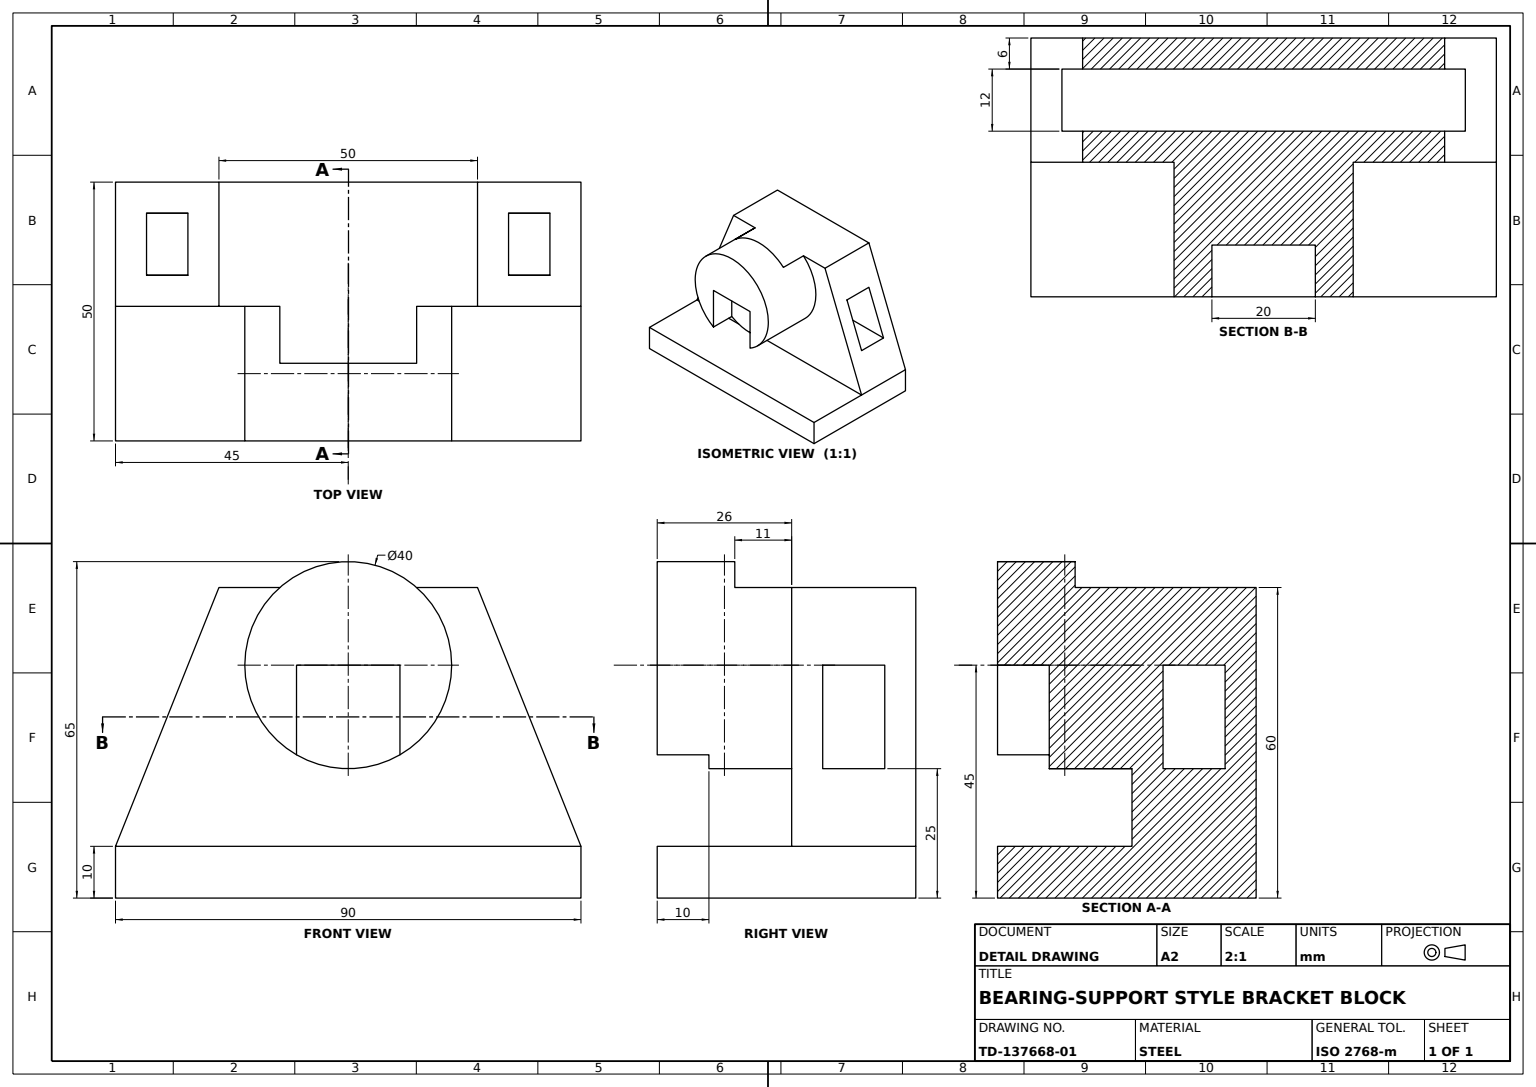
from build123d import *

# Parameters (mm, degrees)
SUPPORT_UPRIGHT_DEPTH      = 24
BASE_PLATE_SKETCH_W        = 90
BASE_PLATE_SKETCH_H        = 10
BASE_PLATE_DEPTH           = 50
BEARING_BOSS_SKETCH_R      = 20
BEARING_BOSS_40_DEPTH      = 26
BOSS_START                 = -10
BOSS_SLOT_CUT_DEPTH        = 10
BOSS_RECESS_CUT_DEPTH      = 11
UPRIGHT_WINDOW_SKETCH_W    = 12
UPRIGHT_WINDOW_SKETCH_H    = 20
UPRIGHT_WINDOW_12X20_DEPTH = 122.757956619


with BuildPart() as part:
    # Support Upright Sketch → Support Upright (new body)
    with BuildSketch(Plane.XY):
        Polygon((0, 10), (20, 60), (70, 60), (90, 10), align=None)
    extrude(amount=SUPPORT_UPRIGHT_DEPTH)

    # Base Plate Sketch → Base Plate (add)
    with BuildSketch(Plane.XY):
        with Locations((45, 5)):
            Rectangle(BASE_PLATE_SKETCH_W, BASE_PLATE_SKETCH_H)
    extrude(amount=BASE_PLATE_DEPTH)

    # Bearing Boss Sketch → Bearing Boss Ø40 (add)
    with BuildSketch(Plane.XY.offset(24)):
        with Locations(Location((45, 45, 0), (0, 0, 131.409622109))):
            Circle(BEARING_BOSS_SKETCH_R)
    extrude(amount=BEARING_BOSS_40_DEPTH)

    # Boss Slot Sketch → Boss Slot Cut (cut)
    with BuildSketch(Plane.XY.offset(50).offset(BOSS_START)):
        with BuildLine():
            Line((35, 45), (55, 45))
            Line((55, 45), (55, 27.679491924))
            ThreePointArc((55, 27.679491924), (45, 25), (35, 27.679491924))
            Line((35, 27.679491924), (35, 45))
        make_face()
    extrude(amount=BOSS_SLOT_CUT_DEPTH, mode=Mode.SUBTRACT)

    # Boss Recess Sketch → Boss Recess Cut (cut)
    with BuildSketch(Plane(origin=(0, 0, 24), x_dir=(-1, 0, 0), z_dir=(0, 0, -1))):
        with BuildLine():
            Line((-58.228756555, 60), (-31.771243445, 60))
            ThreePointArc((-31.771243445, 60), (-45, 65), (-58.228756555, 60))
        make_face()
    extrude(amount=-BOSS_RECESS_CUT_DEPTH, mode=Mode.SUBTRACT)

    # Upright Window Sketch → Upright Window 12x20 (cut, through all)
    with BuildSketch(Plane(origin=(90, 0, 0), x_dir=(0, 0, -1), z_dir=(1, 0, 0))):
        with Locations((-12, 35)):
            Rectangle(UPRIGHT_WINDOW_SKETCH_W, UPRIGHT_WINDOW_SKETCH_H)
    extrude(amount=-UPRIGHT_WINDOW_12X20_DEPTH, mode=Mode.SUBTRACT)


solid = part.part
